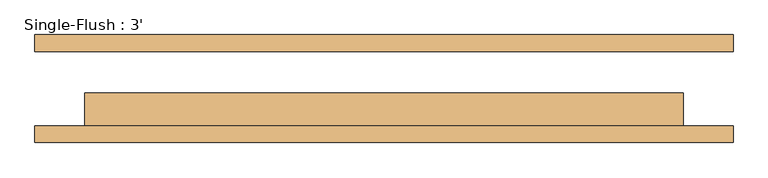
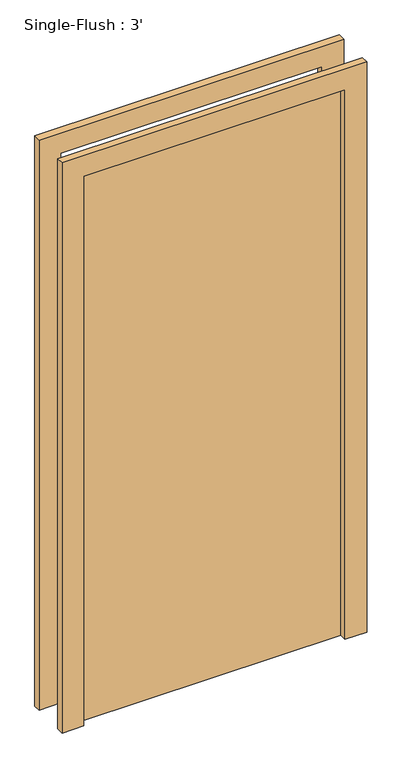
"""IFC4 building model written with IfcOpenShell, lengths in millimetres: door geometry, Single-Flush : 3'."""

from ifc_helpers import new_model, si_unit, frame, origin, origin_with_axes, place, context, project, spatial, polyline, outline, extrude, source, transform, mapped, element, save


def single_flush_3_5e62189b(model_context):
    return source(origin(), model_context, "Body", "SweptSolid", [
        extrude(outline(polyline([(2108.2, -533.4), (0.0, -533.4), (0.0, -457.2), (2032.0, -457.2), (2032.0, 457.2), (0.0, 457.2), (0.0, 533.4), (2108.2, 533.4), (2108.2, -533.4)])), frame((0.0, -82.55, 0.0), z_axis=(0.0, 1.0, 0.0), x_axis=(0.0, 0.0, 1.0)), (0.0, 0.0, 1.0), 25.4),
        extrude(outline(polyline([(2108.2, 533.4), (2108.2, -533.4), (0.0, -533.4), (0.0, -457.2), (2032.0, -457.2), (2032.0, 457.2), (0.0, 457.2), (0.0, 533.4), (2108.2, 533.4)])), frame((0.0, 57.15, 0.0), z_axis=(0.0, 1.0, 0.0), x_axis=(0.0, 0.0, 1.0)), (0.0, 0.0, 1.0), 25.4),
        extrude(outline(polyline([(457.2, -6.35), (457.2, -57.15), (-457.2, -57.15), (-457.2, -6.35), (457.2, -6.35)])), origin_with_axes(), (0.0, 0.0, 1.0), 2032.0),
    ])


if __name__ == "__main__":
    model = new_model("IFC4")
    model_context = context("Model", 3, world=origin())
    ifc_project = project(units=[si_unit("LENGTHUNIT", "METRE", prefix="MILLI")], contexts=[model_context])
    site = spatial("IfcSite", under=ifc_project)
    building = spatial("IfcBuilding", under=site)
    placement = place(None, origin())
    single_flush_3_shape = single_flush_3_5e62189b(model_context)
    element("IfcDoor", 1, ObjectType="Single-Flush : 3'", at=placement, inside=building, context=model_context, shape_type="MappedRepresentation", body=[
        mapped(single_flush_3_shape, transform((0.0, 0.0, 0.0), x_axis=(1.0, 0.0, 0.0), y_axis=(0.0, 1.0, 0.0), z_axis=(0.0, 0.0, 1.0))),
    ])
    save(model, "model.ifc")

# Revit data of these elements
# Type "Single-Flush : 3'"
#   Type Mark = "8"
#   Construction Type Id = "MDOOR"
#   Assembly Code = "C1020"
#   Analytic Construction = "Metal"
#   Thickness = 0' - 2"
#   Heat Transfer Coefficient (U) = 0.651978 BTU/(h·ft²·°F)
#   Height = 6' - 8"
#   Trim Projection Ext = 0' - 1"
#   Trim Projection Int = 0' - 1"
#   Trim Width = 0' - 3"
#   Width = 3' - 0"
#   Define Thermal Properties by = 1
#   Door Material = Door - Panel
#   Frame Material = Door - Frame
#   Visual Light Transmittance = 0
#   Solar Heat Gain Coefficient = 0
#   Function = (empty or 0)
#   Wall Closure = (empty or 0)
# Element 1 (IfcDoor, "Single-Flush : 3'")
#   Materials on its faces: "Door - Frame", "Door - Panel"
# Materials
#   "Door - Panel": class "Wood", colour RGB 210 159 95, transparency 0, Cost = 0
#   "Door - Frame": colour RGB 118 70 51, transparency 0, Cost = 0
